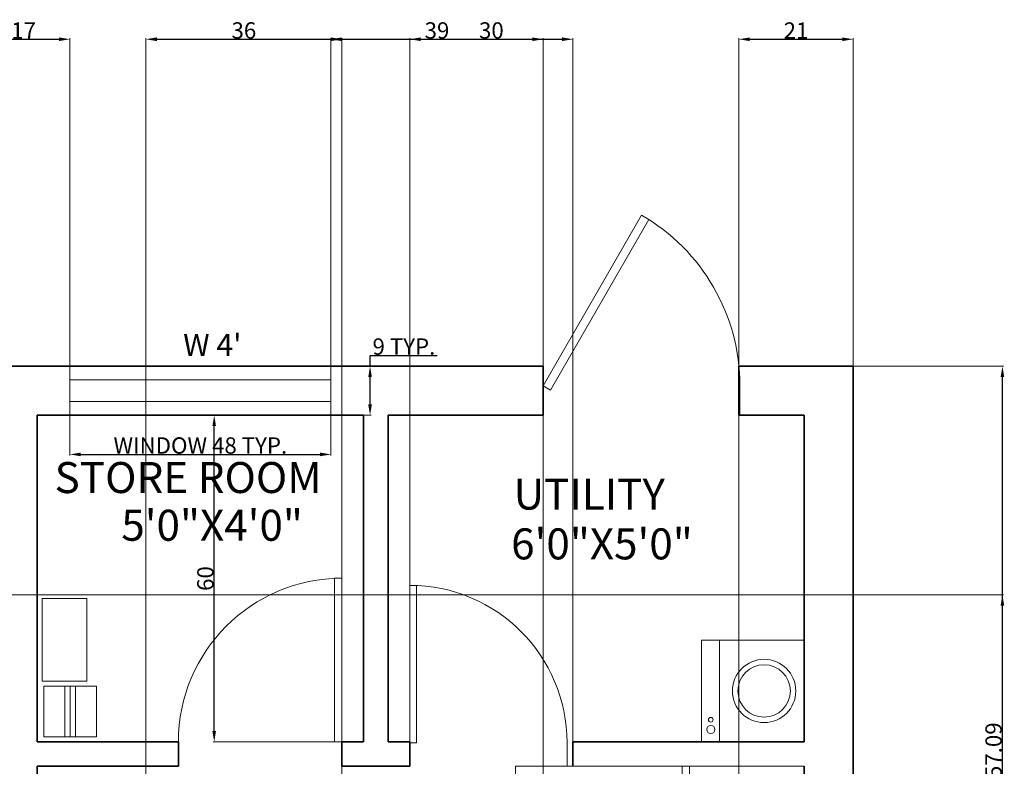
# Model space of a CAD drawing. Units: feet. Extents: x -297 to 770, y -228 to 625.
# Tile 14 of 14: x 589 to 770, y 233 to 371. Entities that reach past the tile are written whole.
import ezdxf

# ---------------------------------------------------------------- set-up
doc = ezdxf.new("R2010")
doc.units = ezdxf.units.FT
doc.header["$MEASUREMENT"] = 0
for name, color, linetype, lineweight in [('A-ANNO-DIMS', 2, 'Continuous', 18), ('A-ANNO-TEXT', 7, 'Continuous', 18), ('A-AREA-IDEN', 7, 'Continuous', 25), ('A-EQPM', 8, 'Continuous', 13), ('A-FLOR-CASE', 8, 'Continuous', 18), ('A-FLOR-FIXT', 8, 'Continuous', 18), ('A-WALL', 7, 'Continuous', 35), ('doors', 30, 'Continuous', 18), ('windows', 30, 'Continuous', 18)]:
    doc.layers.add(name, color=color, linetype=linetype, lineweight=lineweight)
doc.styles.add('Annotative', font='arial.ttf')
doc.styles.get("Standard").update_dxf_attribs({"font": 'arial.ttf'})
doc.dimstyles.get("Standard").update_dxf_attribs({"dimtxt": 3, "dimasz": 2, "dimexe": 0.18, "dimexo": 0.0625, "dimgap": 0.09, "dimtad": 1, "dimtoh": 1, "dimdec": 1, "dimzin": 0, "dimdsep": 46, "dimlunit": 3, "dimtxsty": 'Standard', "dimcen": 0, "dimclre": 256, "dimadec": 0, "dimazin": 0, "dimtfac": 1, "dimtdec": 1, "dimtofl": 0, "dimtmove": 0, "dimatfit": 3, "dimfxl": 1, "dimtolj": 1, "dimtzin": 0, "dimlwe": -1, "dimarcsym": 0})

# ---------------------------------------------------------------- blocks, each defined once
blk = doc.blocks.new('*U2')
for p, q in [((0, 0), (0, -6)), ((-40, 0), (-40, -6))]:
    blk.add_line(p, q)
blk.add_lwpolyline([(0, 0), (0, 40), (-1.75, 40), (-1.75, 0)], close=True)
blk.add_arc((0, 0), 40, 90, 180)
blk = doc.blocks.new('*U6')
for p, q in [((0, 0), (0, -6)), ((40, 0), (40, -6))]:
    blk.add_line(p, q)
blk.add_lwpolyline([(0, 0), (0, 40), (1.75, 40), (1.75, 0)], close=True)
blk.add_arc((0, 0), 40, 0, 90)
blk = doc.blocks.new('*U3')
for p, q in [((0, 0), (0, -6)), ((40, 0), (40, -6))]:
    blk.add_line(p, q)
blk.add_lwpolyline([(0, 0), (20, 34.64), (21.52, 33.77), (1.52, -0.88)], close=True)
blk.add_arc((0, 0), 40, 0, 60)
blk = doc.blocks.new('WIN-4FT')
for p, q in [((48, 9), (0, 9)), ((0, 9), (0, 0)), ((48, 0), (48, 9)), ((0, 6.5), (48, 6.5)), ((0, 2.5), (48, 2.5)), ((0, 0), (48, 0))]:
    blk.add_line(p, q)
blk = doc.blocks.new('*D21')
at = {"layer": 'A-ANNO-DIMS', "transparency": 16777216}
for p, q in [((598.16, 297.9), (598.16, 290.58)), ((646.16, 297.9), (646.16, 290.58))]:
    blk.add_line(p, q, dxfattribs=at)
at = {"layer": 'A-ANNO-DIMS', "color": 0, "lineweight": -2, "transparency": 16777216}
blk.add_line((600.16, 290.76), (644.16, 290.76), dxfattribs=at)
at = {"layer": 'A-ANNO-DIMS', "color": 0, "transparency": 16777216}
for points in [[(600.16, 291.1), (600.16, 290.43), (598.16, 290.76)], [(644.16, 291.1), (644.16, 290.43), (646.16, 290.76)]]:
    blk.add_solid(points, dxfattribs=at)
at = {"layer": 'Defpoints', "color": 0, "transparency": 16777216}
for p in [(598.16, 297.96), (646.16, 297.96), (646.16, 290.76)]:
    blk.add_point(p, dxfattribs=at)
at = {"layer": 'A-ANNO-DIMS', "color": 0, "transparency": 16777216, "insert": (622.16, 292.4), "char_height": 3, "attachment_point": 5}
blk.add_mtext('\\A1;WINDOW 48 TYP.', dxfattribs=at)
blk = doc.blocks.new('*D22')
at = {"layer": 'A-ANNO-DIMS', "color": 0, "lineweight": -2, "transparency": 16777216}
for p, q in [((653.36, 306.96), (653.36, 308.96)), ((653.36, 308.96), (665.72, 308.96)), ((653.36, 299.96), (653.36, 304.96))]:
    blk.add_line(p, q, dxfattribs=at)
at = {"layer": 'A-ANNO-DIMS', "transparency": 16777216}
for p, q in [((646.22, 306.96), (653.54, 306.96)), ((646.22, 297.96), (653.54, 297.96))]:
    blk.add_line(p, q, dxfattribs=at)
at = {"layer": 'A-ANNO-DIMS', "color": 0, "transparency": 16777216}
for points in [[(653.02, 304.96), (653.69, 304.96), (653.36, 306.96)], [(653.02, 299.96), (653.69, 299.96), (653.36, 297.96)]]:
    blk.add_solid(points, dxfattribs=at)
at = {"layer": 'Defpoints', "color": 0, "transparency": 16777216}
for p in [(646.16, 306.96), (653.36, 306.96), (646.16, 297.96)]:
    blk.add_point(p, dxfattribs=at)
at = {"layer": 'A-ANNO-DIMS', "color": 0, "transparency": 16777216, "insert": (659.58, 310.58), "char_height": 3, "attachment_point": 5}
blk.add_mtext('\\A1;9 TYP.', dxfattribs=at)
blk = doc.blocks.new('*D44')
at = {"layer": 'A-ANNO-DIMS', "transparency": 16777216}
for p, q in [((742.22, 306.96), (769.79, 306.96)), ((742.22, -200.04), (769.79, -200.04))]:
    blk.add_line(p, q, dxfattribs=at)
at = {"layer": 'A-ANNO-DIMS', "color": 0, "lineweight": -2, "transparency": 16777216}
blk.add_line((769.61, -198.04), (769.61, 304.96), dxfattribs=at)
at = {"layer": 'A-ANNO-DIMS', "color": 0, "transparency": 16777216}
for points in [[(769.27, 304.96), (769.94, 304.96), (769.61, 306.96)], [(769.27, -198.04), (769.94, -198.04), (769.61, -200.04)]]:
    blk.add_solid(points, dxfattribs=at)
at = {"layer": 'Defpoints', "color": 0, "transparency": 16777216}
for p in [(742.16, 306.96), (769.61, 306.96), (742.16, -200.04)]:
    blk.add_point(p, dxfattribs=at)
at = {"layer": 'A-ANNO-DIMS', "color": 0, "transparency": 16777216, "insert": (767.98, 53.46), "char_height": 3, "attachment_point": 5, "rotation": 90}
blk.add_mtext('\\A1;507', dxfattribs=at)
blk = doc.blocks.new('*D48')
at = {"layer": 'A-ANNO-DIMS', "transparency": 16777216}
for p, q in [((581.16, 307.03), (581.16, 367.22)), ((598.16, 307.03), (598.16, 367.22))]:
    blk.add_line(p, q, dxfattribs=at)
at = {"layer": 'A-ANNO-DIMS', "color": 0, "lineweight": -2, "transparency": 16777216}
blk.add_line((583.16, 367.04), (596.16, 367.04), dxfattribs=at)
at = {"layer": 'A-ANNO-DIMS', "color": 0, "transparency": 16777216}
for points in [[(583.16, 367.38), (583.16, 366.71), (581.16, 367.04)], [(596.16, 367.38), (596.16, 366.71), (598.16, 367.04)]]:
    blk.add_solid(points, dxfattribs=at)
at = {"layer": 'Defpoints', "color": 0, "transparency": 16777216}
for p in [(598.16, 367.04), (581.16, 306.96), (598.16, 306.96)]:
    blk.add_point(p, dxfattribs=at)
at = {"layer": 'A-ANNO-DIMS', "color": 0, "transparency": 16777216, "insert": (589.66, 368.64), "char_height": 3, "attachment_point": 5}
blk.add_mtext('\\A1;17', dxfattribs=at)
blk = doc.blocks.new('*D49')
at = {"layer": 'A-ANNO-DIMS', "transparency": 16777216}
for p, q in [((646.16, 307.03), (646.16, 367.22)), ((685.16, 307.03), (685.16, 367.22))]:
    blk.add_line(p, q, dxfattribs=at)
at = {"layer": 'A-ANNO-DIMS', "color": 0, "lineweight": -2, "transparency": 16777216}
blk.add_line((648.16, 367.04), (683.16, 367.04), dxfattribs=at)
at = {"layer": 'A-ANNO-DIMS', "color": 0, "transparency": 16777216}
for points in [[(648.16, 367.38), (648.16, 366.71), (646.16, 367.04)], [(683.16, 367.38), (683.16, 366.71), (685.16, 367.04)]]:
    blk.add_solid(points, dxfattribs=at)
at = {"layer": 'Defpoints', "color": 0, "transparency": 16777216}
for p in [(685.16, 367.04), (646.16, 306.96), (685.16, 306.96)]:
    blk.add_point(p, dxfattribs=at)
at = {"layer": 'A-ANNO-DIMS', "color": 0, "transparency": 16777216, "insert": (665.66, 368.66), "char_height": 3, "attachment_point": 5}
blk.add_mtext('\\A1;39', dxfattribs=at)
blk = doc.blocks.new('*D50')
at = {"layer": 'A-ANNO-DIMS', "transparency": 16777216}
for p, q in [((721.16, 307.03), (721.16, 367.22)), ((742.16, 307.03), (742.16, 367.22))]:
    blk.add_line(p, q, dxfattribs=at)
at = {"layer": 'A-ANNO-DIMS', "color": 0, "lineweight": -2, "transparency": 16777216}
blk.add_line((723.16, 367.04), (740.16, 367.04), dxfattribs=at)
at = {"layer": 'A-ANNO-DIMS', "color": 0, "transparency": 16777216}
for points in [[(723.16, 367.38), (723.16, 366.71), (721.16, 367.04)], [(740.16, 367.38), (740.16, 366.71), (742.16, 367.04)]]:
    blk.add_solid(points, dxfattribs=at)
at = {"layer": 'Defpoints', "color": 0, "transparency": 16777216}
for p in [(742.16, 367.04), (721.16, 306.96), (742.16, 306.96)]:
    blk.add_point(p, dxfattribs=at)
at = {"layer": 'A-ANNO-DIMS', "color": 0, "transparency": 16777216, "insert": (731.66, 368.64), "char_height": 3, "attachment_point": 5}
blk.add_mtext('\\A1;21', dxfattribs=at)
blk = doc.blocks.new('*D63')
at = {"layer": 'A-ANNO-DIMS', "transparency": 16777216}
for p, q in [((612.16, 113.53), (612.16, 367.22)), ((648.16, 113.53), (648.16, 367.22))]:
    blk.add_line(p, q, dxfattribs=at)
at = {"layer": 'A-ANNO-DIMS', "color": 0, "lineweight": -2, "transparency": 16777216}
blk.add_line((614.16, 367.04), (646.16, 367.04), dxfattribs=at)
at = {"layer": 'A-ANNO-DIMS', "color": 0, "transparency": 16777216}
for points in [[(614.16, 367.38), (614.16, 366.71), (612.16, 367.04)], [(646.16, 367.38), (646.16, 366.71), (648.16, 367.04)]]:
    blk.add_solid(points, dxfattribs=at)
at = {"layer": 'Defpoints', "color": 0, "transparency": 16777216}
for p in [(648.16, 367.04), (612.16, 113.46), (648.16, 113.46)]:
    blk.add_point(p, dxfattribs=at)
at = {"layer": 'A-ANNO-DIMS', "color": 0, "transparency": 16777216, "insert": (630.16, 368.66), "char_height": 3, "attachment_point": 5}
blk.add_mtext('\\A1;36', dxfattribs=at)
blk = doc.blocks.new('*D65')
at = {"layer": 'A-ANNO-DIMS', "transparency": 16777216}
for p, q in [((660.66, 238.03), (660.66, 367.22)), ((690.66, 238.03), (690.66, 367.22))]:
    blk.add_line(p, q, dxfattribs=at)
at = {"layer": 'A-ANNO-DIMS', "color": 0, "lineweight": -2, "transparency": 16777216}
blk.add_line((662.66, 367.04), (688.66, 367.04), dxfattribs=at)
at = {"layer": 'A-ANNO-DIMS', "color": 0, "transparency": 16777216}
for points in [[(662.66, 367.38), (662.66, 366.71), (660.66, 367.04)], [(688.66, 367.38), (688.66, 366.71), (690.66, 367.04)]]:
    blk.add_solid(points, dxfattribs=at)
at = {"layer": 'Defpoints', "color": 0, "transparency": 16777216}
for p in [(690.66, 367.04), (660.66, 237.96), (690.66, 237.96)]:
    blk.add_point(p, dxfattribs=at)
at = {"layer": 'A-ANNO-DIMS', "color": 0, "transparency": 16777216, "insert": (675.66, 368.66), "char_height": 3, "attachment_point": 5}
blk.add_mtext('\\A1;30', dxfattribs=at)
blk = doc.blocks.new('*D68')
at = {"layer": 'A-ANNO-DIMS', "transparency": 16777216}
for p, q in [((685.16, 306.9), (685.16, -227.67)), ((721.16, 306.9), (721.16, -227.67))]:
    blk.add_line(p, q, dxfattribs=at)
at = {"layer": 'A-ANNO-DIMS', "color": 0, "lineweight": -2, "transparency": 16777216}
blk.add_line((687.16, -227.49), (719.16, -227.49), dxfattribs=at)
at = {"layer": 'A-ANNO-DIMS', "color": 0, "transparency": 16777216}
for points in [[(687.16, -227.15), (687.16, -227.82), (685.16, -227.49)], [(719.16, -227.15), (719.16, -227.82), (721.16, -227.49)]]:
    blk.add_solid(points, dxfattribs=at)
at = {"layer": 'Defpoints', "color": 0, "transparency": 16777216}
for p in [(685.16, 306.96), (721.16, 306.96), (721.16, -227.49)]:
    blk.add_point(p, dxfattribs=at)
at = {"layer": 'A-ANNO-DIMS', "color": 0, "transparency": 16777216, "insert": (703.16, -225.86), "char_height": 3, "attachment_point": 5}
blk.add_mtext('\\A1;36', dxfattribs=at)
blk = doc.blocks.new('*D75')
at = {"layer": 'A-ANNO-DIMS', "transparency": 16777216}
for p, q in [((471.75, 264.96), (769.79, 264.96)), ((471.75, 207.87), (769.79, 207.87))]:
    blk.add_line(p, q, dxfattribs=at)
at = {"layer": 'A-ANNO-DIMS', "color": 0, "lineweight": -2, "transparency": 16777216}
blk.add_line((769.61, 209.87), (769.61, 262.96), dxfattribs=at)
at = {"layer": 'A-ANNO-DIMS', "color": 0, "transparency": 16777216}
for points in [[(769.27, 262.96), (769.94, 262.96), (769.61, 264.96)], [(769.27, 209.87), (769.94, 209.87), (769.61, 207.87)]]:
    blk.add_solid(points, dxfattribs=at)
at = {"layer": 'Defpoints', "color": 0, "transparency": 16777216}
for p in [(471.69, 264.96), (769.61, 264.96), (471.69, 207.87)]:
    blk.add_point(p, dxfattribs=at)
at = {"layer": 'A-ANNO-DIMS', "color": 0, "transparency": 16777216, "insert": (767.98, 236.42), "char_height": 3, "attachment_point": 5, "rotation": 90}
blk.add_mtext('\\A1;57.09', dxfattribs=at)
blk = doc.blocks.new('*D85')
at = {"layer": 'A-ANNO-DIMS', "transparency": 16777216}
for p, q in [((652.09, 297.96), (624.53, 297.96)), ((652.09, 237.96), (624.53, 237.96))]:
    blk.add_line(p, q, dxfattribs=at)
at = {"layer": 'A-ANNO-DIMS', "color": 0, "lineweight": -2, "transparency": 16777216}
blk.add_line((624.71, 239.96), (624.71, 295.96), dxfattribs=at)
at = {"layer": 'A-ANNO-DIMS', "color": 0, "transparency": 16777216}
for points in [[(624.37, 295.96), (625.04, 295.96), (624.71, 297.96)], [(624.37, 239.96), (625.04, 239.96), (624.71, 237.96)]]:
    blk.add_solid(points, dxfattribs=at)
at = {"layer": 'Defpoints', "color": 0, "transparency": 16777216}
for p in [(624.71, 297.96), (652.16, 297.96), (652.16, 237.96)]:
    blk.add_point(p, dxfattribs=at)
at = {"layer": 'A-ANNO-DIMS', "color": 0, "transparency": 16777216, "insert": (623.08, 267.96), "char_height": 3, "attachment_point": 5, "rotation": 90}
blk.add_mtext('\\A1;60', dxfattribs=at)

msp = doc.modelspace()

# ---------------------------------------------------------------- linework, layer by layer
at = {"layer": 'A-EQPM'}
msp.add_line((717.576, 256.646), (717.576, 237.963), dxfattribs=at)
msp.add_lwpolyline([(733.155, 237.963), (714.256, 237.963), (714.256, 256.646), (733.155, 256.646)], close=True, dxfattribs=at)
for centre, radius in [((725.798, 247.304), 5.82), ((725.798, 247.304), 4.82), ((715.996, 240.218), 0.745), ((715.996, 242.019), 0.435)]:
    msp.add_circle(centre, radius, dxfattribs=at)
at = {"layer": 'A-FLOR-CASE'}
for p, q in [((597.232, 248.164), (597.232, 238.86)), ((598.232, 248.164), (598.232, 238.86)), ((599.232, 248.164), (599.232, 238.86)), ((680.083, 217.736), (680.083, 233.463)), ((680.083, 233.463), (733.158, 233.463)), ((733.155, 113.516), (733.155, 233.463))]:
    msp.add_line(p, q, dxfattribs=at)
for points in [[(593.094, 249.084), (601.306, 249.084), (601.306, 264.3), (593.094, 264.3)], [(593.384, 238.86), (603.08, 238.86), (603.08, 248.164), (593.384, 248.164)]]:
    msp.add_lwpolyline(points, close=True, dxfattribs=at)
at = {"layer": 'A-FLOR-FIXT'}
for p, q in [((710.749, 230.375), (710.749, 233.463)), ((712.053, 230.375), (712.053, 233.463))]:
    msp.add_line(p, q, dxfattribs=at)
at = {"layer": 'A-WALL'}
for p, q in [((685.155, 297.963), (685.155, 306.963)), ((721.155, 297.963), (721.155, 306.963)), ((742.155, -200.037), (742.155, 306.963)), ((592.155, 237.963), (592.155, 297.963)), ((652.155, 237.963), (652.155, 297.963)), ((656.655, 237.963), (656.655, 297.963)), ((618.155, 237.963), (592.155, 237.963)), ((618.155, 233.463), (618.155, 237.963)), ((652.155, 237.963), (648.155, 237.963)), ((648.155, 233.463), (648.155, 237.963)), ((660.655, 237.963), (656.655, 237.963)), ((660.655, 233.463), (660.655, 237.963)), ((733.155, 237.963), (690.655, 237.963)), ((690.655, 233.463), (690.655, 237.963)), ((592.155, 233.463), (592.155, 113.463)), ((618.155, 233.463), (592.155, 233.463)), ((660.655, 233.463), (648.155, 233.463))]:
    msp.add_line(p, q, dxfattribs=at)
for points in [[(685.155, 306.963), (382.155, 306.963), (382.155, -173.037), (556.155, -173.037)], [(742.155, 306.963), (721.155, 306.963)], [(652.155, 297.963), (592.155, 297.963)], [(685.155, 297.963), (656.655, 297.963)], [(733.155, 237.963), (733.155, 297.963), (721.155, 297.963)], [(733.155, 113.463), (733.155, 233.463)]]:
    msp.add_lwpolyline(points, dxfattribs=at)

# ---------------------------------------------------------------- block references
at = {"layer": 'doors'}
for name, p, xscale, yscale, zscale in [('*U3', (685.155, 303.393), 0.9049851433260272, 0.9049851433260272, 0.9049851433260272), ('*U2', (648.155, 237.968), 0.7508659147465452, 0.7508659147465452, 0.7508659147465452), ('*U6', (660.655, 237.799), 0.7226421799388985, 0.7226421799388985, 0.7226421799388985)]:
    msp.add_blockref(name, p, dxfattribs=dict(at, xscale=xscale, yscale=yscale, zscale=zscale))
at = {"layer": 'windows'}
msp.add_blockref('WIN-4FT', (598.155, 297.963), dxfattribs=at)

# ---------------------------------------------------------------- texts
at = {"layer": 'A-ANNO-TEXT', "style": 'Annotative'}
msp.add_text("W 4'", height=4.0626, dxfattribs=at).set_placement((619, 308.849))
at = {"layer": 'A-AREA-IDEN', "style": 'Annotative'}
for s, p in [('STORE ROOM', (595.365, 283.668)), ('UTILITY', (679.748, 280.629)), ('5\'0"X4\'0"', (607.626, 274.899)), ('6\'0"X5\'0"', (679.291, 271.479))]:
    msp.add_text(s, height=5.696, dxfattribs=at).set_placement(p)

# ---------------------------------------------------------------- dimensions: what is measured, and where the dimension line sits
at = {"layer": 'A-ANNO-DIMS'}
for base, p1, p2, picture, middle in [((598.155, 367.042), (581.155, 306.963), (598.155, 306.963), '*D48', (589.655, 368.638)), ((648.155, 367.042), (612.155, 113.463), (648.155, 113.463), '*D63', (630.155, 368.665)), ((685.155, 367.042), (646.155, 306.963), (685.155, 306.963), '*D49', (665.655, 368.665)), ((690.655, 367.042), (660.655, 237.963), (690.655, 237.963), '*D65', (675.655, 368.665)), ((742.155, 367.042), (721.155, 306.963), (742.155, 306.963), '*D50', (731.655, 368.638)), ((721.155, -227.487), (685.155, 306.963), (721.155, 306.963), '*D68', (703.155, -225.865))]:
    dim = msp.add_linear_dim(base=base, p1=p1, p2=p2, dimstyle='Standard', override={"dimdec": 0, "dimlfac": 1, "dimrnd": 0, "dimzin": 0, "dimdsep": 46, "dimlunit": 2}, dxfattribs=at)
    dim.commit()
    dim.dimension.update_dxf_attribs({"geometry": picture, "text_midpoint": middle})
dim = msp.add_linear_dim(base=(653.355, 306.963), p1=(646.155, 297.963), p2=(646.155, 306.963), angle=90, text='<> TYP.', dimstyle='Standard', override={"dimdec": 0, "dimlfac": 1, "dimrnd": 0, "dimzin": 0, "dimdsep": 46, "dimlunit": 2}, dxfattribs=at)
dim.commit()
dim.dimension.update_dxf_attribs({"geometry": '*D22', "text_midpoint": (659.581, 310.584)})
for base, p1, p2, override, picture, middle in [((769.605, 306.963), (742.155, -200.037), (742.155, 306.963), {"dimdec": 0, "dimlfac": 1, "dimrnd": 0, "dimzin": 0, "dimdsep": 46, "dimlunit": 2}, '*D44', (767.984, 53.463)), ((624.705, 297.963), (652.155, 237.963), (652.155, 297.963), {"dimdec": 0, "dimlfac": 1, "dimrnd": 0, "dimzin": 0, "dimdsep": 46, "dimlunit": 2}, '*D85', (623.084, 267.963)), ((769.605, 264.961), (471.691, 207.869), (471.691, 264.961), {"dimdec": 2, "dimlfac": 1, "dimrnd": 0, "dimzin": 0, "dimdsep": 46, "dimlunit": 2}, '*D75', (767.984, 236.415))]:
    dim = msp.add_linear_dim(base=base, p1=p1, p2=p2, angle=90, dimstyle='Standard', override=override, dxfattribs=at)
    dim.commit()
    dim.dimension.update_dxf_attribs({"geometry": picture, "text_midpoint": middle})
dim = msp.add_linear_dim(base=(646.155, 290.763), p1=(598.155, 297.963), p2=(646.155, 297.963), text='WINDOW <> TYP.', dimstyle='Standard', override={"dimdec": 0, "dimlfac": 1, "dimrnd": 0, "dimzin": 0, "dimdsep": 46, "dimlunit": 2}, dxfattribs=at)
dim.commit()
dim.dimension.update_dxf_attribs({"geometry": '*D21', "text_midpoint": (622.155, 292.405)})

doc.saveas('drawing.dxf')
